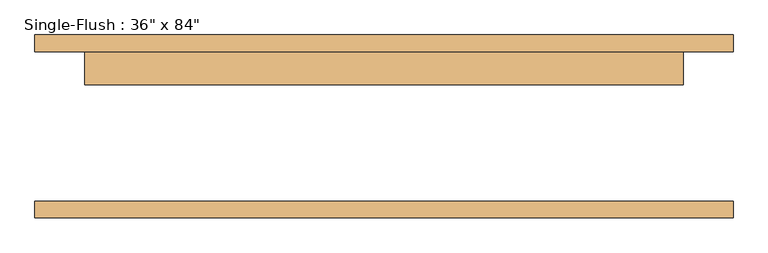
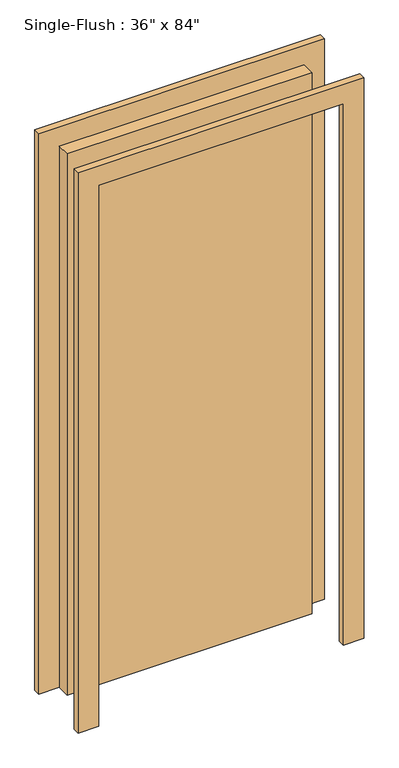
"""IFC4 building model written with IfcOpenShell, lengths in millimetres: door geometry."""

from ifc_helpers import new_model, si_unit, frame, origin, origin_with_axes, place, context, project, spatial, polyline, outline, extrude, source, transform, mapped, element, save


def door_0ca8825f(model_context):
    return source(origin(), model_context, "Body", "SweptSolid", [
        extrude(outline(polyline([(2209.8, -533.4), (0.0, -533.4), (0.0, -457.2), (2133.6, -457.2), (2133.6, 457.2), (0.0, 457.2), (0.0, 533.4), (2209.8, 533.4), (2209.8, -533.4)])), frame((0.0, 114.3, 0.0), z_axis=(0.0, 1.0, 0.0), x_axis=(0.0, 0.0, 1.0)), (0.0, 0.0, 1.0), 25.4),
        extrude(outline(polyline([(2209.8, 533.4), (2209.8, -533.4), (0.0, -533.4), (0.0, -457.2), (2133.6, -457.2), (2133.6, 457.2), (0.0, 457.2), (0.0, 533.4), (2209.8, 533.4)])), frame((0.0, -139.7, 0.0), z_axis=(0.0, 1.0, 0.0), x_axis=(0.0, 0.0, 1.0)), (0.0, 0.0, 1.0), 25.4),
        extrude(outline(polyline([(457.2, 63.5), (-457.2, 63.5), (-457.2, 114.3), (457.2, 114.3), (457.2, 63.5)])), origin_with_axes(), (0.0, 0.0, 1.0), 2133.6),
    ])


if __name__ == "__main__":
    model = new_model("IFC4")
    model_context = context("Model", 3, world=origin())
    ifc_project = project(units=[si_unit("LENGTHUNIT", "METRE", prefix="MILLI")], contexts=[model_context])
    site = spatial("IfcSite", under=ifc_project)
    building = spatial("IfcBuilding", under=site)
    placement = place(None, origin())
    door_shape = door_0ca8825f(model_context)
    element("IfcDoor", 1, ObjectType="Single-Flush : 36\" x 84\"", at=placement, inside=building, context=model_context, shape_type="MappedRepresentation", body=[
        mapped(door_shape, transform((0.0, 0.0, 0.0), x_axis=(1.0, 0.0, 0.0), y_axis=(0.0, 1.0, 0.0), z_axis=(0.0, 0.0, 1.0))),
    ])
    save(model, "model.ifc")

# Revit data of these elements
# Type "Single-Flush : 36\" x 84\""
#   Type Mark = "1"
#   Construction Type Id = "MDOOR"
#   Assembly Code = "C1020"
#   Analytic Construction = "Metal"
#   Thickness = 0' - 2"
#   Heat Transfer Coefficient (U) = 0.651978 BTU/(h·ft²·°F)
#   Height = 7' - 0"
#   Trim Projection Ext = 0' - 1"
#   Trim Projection Int = 0' - 1"
#   Trim Width = 0' - 3"
#   Width = 3' - 0"
#   Define Thermal Properties by = 1
#   Define Thermal Properties by = 1
#   Door Material = Door - Panel
#   Frame Material = Door - Frame
#   Visual Light Transmittance = 0
#   Solar Heat Gain Coefficient = 0
#   Function = (empty or 0)
#   Wall Closure = (empty or 0)
# Element 1 (IfcDoor, "Single-Flush : 36\" x 84\"")
#   Materials on its faces: "Door - Frame", "Door - Panel"
# Materials
#   "Door - Panel": class "Wood", colour RGB 210 159 95, transparency 0, Cost = 0
#   "Door - Frame": colour RGB 118 70 51, transparency 0, Cost = 0
